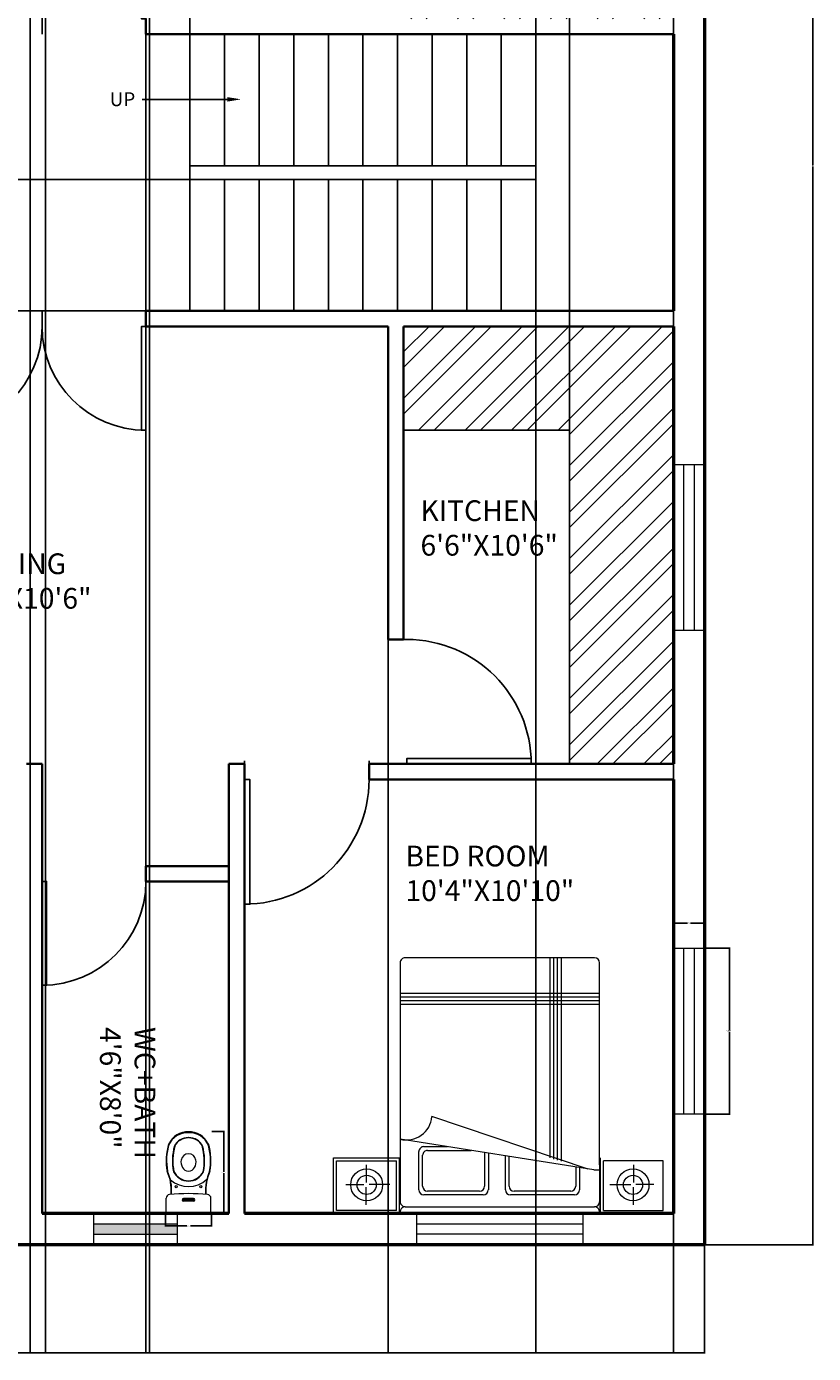
# Model space of a CAD drawing. Units: feet. Extents: x 2664 to 3060, y 1318 to 2005.
# Tile 2 of 5: x 2832 to 3060, y 1318 to 1702. Entities that reach past the tile are written whole.
import ezdxf
from ezdxf import colors
from ezdxf.entities.mleader import LeaderData, LeaderLine
from ezdxf.math import Vec2, Vec3

# ---------------------------------------------------------------- set-up
doc = ezdxf.new("R2010")
doc.units = ezdxf.units.FT
for name, color, linetype, lineweight in [('A-ANNO-DIMS', 2, 'Continuous', 18), ('A-ANNO-SYMB', 182, 'Continuous', 18), ('A-AREA-IDEN', 109, 'Continuous', 18), ('A-WALL-EXTR', 130, 'Continuous', 50), ('DOOR', 249, 'Continuous', 25), ('FURNITURE', 240, 'Continuous', 13), ('SANITARY', 50, 'Continuous', 13), ('STAIR', 182, 'Continuous', 25)]:
    doc.layers.add(name, color=color, linetype=linetype, lineweight=lineweight)
for name, color, linetype, lineweight, true_color in [('A-CASE', 41, 'Continuous', 25, 0xf5dd7a), ('A-CASE-PATT', 152, 'Continuous', 13, 0x2776bb), ('A-GLAZ', 222, 'Continuous', 18, 0xd4008b), ('A-VENT-PATT', 219, 'Continuous', 13, 0x642165), ('A-WALL-INTR', 41, 'Continuous', 35, 0xf5dd7a), ('VENT', 95, 'Continuous', 18, 0x46b72a)]:
    doc.layers.add(name, color=color, linetype=linetype, lineweight=lineweight, true_color=true_color)
doc.styles.get("Standard").update_dxf_attribs({"font": 'arial.ttf'})
doc.dimstyles.get("Standard").update_dxf_attribs({"dimtxt": 0.18, "dimasz": 0.18, "dimexe": 0.18, "dimexo": 0.0625, "dimgap": 0.09, "dimtad": 0, "dimtih": 1, "dimtoh": 1, "dimdec": 4, "dimzin": 0, "dimdsep": 46, "dimtxsty": 'Standard', "dimcen": 0.09, "dimadec": 0, "dimazin": 0, "dimtfac": 1, "dimtdec": 4, "dimtofl": 0, "dimtmove": 0, "dimatfit": 3, "dimfxl": 1, "dimtolj": 1, "dimtzin": 0, "dimarcsym": 0})

# ---------------------------------------------------------------- blocks, each defined once
blk = doc.blocks.new('*U4')
for p, q in [((0, 0), (0, 6)), ((40, 0), (40, 6))]:
    blk.add_line(p, q)
blk.add_lwpolyline([(0, 0), (0, -40), (1.75, -40), (1.75, 0)], close=True)
blk.add_arc((0, 0), 40, 270, 0)
blk = doc.blocks.new('*U3')
for p, q in [((0, 0), (0, -6)), ((-40, 0), (-40, -6))]:
    blk.add_line(p, q)
blk.add_lwpolyline([(0, 0), (0, 40), (-1.75, 40), (-1.75, 0)], close=True)
blk.add_arc((0, 0), 40, 90, 180)
blk = doc.blocks.new('*U7')
for p, q in [((0, 0), (0, 6)), ((40, 0), (40, 6))]:
    blk.add_line(p, q)
blk.add_lwpolyline([(0, 0), (0, -40), (1.75, -40), (1.75, 0)], close=True)
blk.add_arc((0, 0), 40, 270, 360)
blk = doc.blocks.new('*U2')
for p, q in [((0, 0), (0, -6)), ((40, 0), (40, -6))]:
    blk.add_line(p, q)
blk.add_lwpolyline([(0, 0), (0, 40), (1.75, 40), (1.75, 0)], close=True)
blk.add_arc((0, 0), 40, 0, 90)
blk = doc.blocks.new('*U6')
for p, q in [((0, 0), (0, 6)), ((40, 0), (40, 6))]:
    blk.add_line(p, q)
blk.add_lwpolyline([(0, 0), (0, -40), (1.75, -40), (1.75, 0)], close=True)
blk.add_arc((0, 0), 40, 270, 0)
blk = doc.blocks.new('BED-DOUBLE-WITH-NIGHTSTANDS')
for p, q in [((-29.54, 0), (-29.54, -16.21)), ((-30.37, -0.95), (-47.65, -0.95)), ((-47.65, -0.95), (-47.65, -15.35)), ((-39.11, -2.58), (-39.11, -7.74)), ((-30.37, -0.95), (-30.37, -15.35)), ((-29.47, -0.05), (-29.47, -16.25)), ((-29.26, -14.16), (-29.26, -3.5)), ((28.27, -0.11), (-29.17, -0.11)), ((26.92, -2.06), (-27.82, -2.06)), ((28.36, -72.65), (28.36, -3.5)), ((28.57, -0.05), (47.65, -0.05)), ((28.57, -0.05), (28.57, -16.25)), ((29.47, -0.95), (46.75, -0.95)), ((29.47, -0.95), (29.47, -15.35)), ((38.21, -2.58), (38.21, -7.74)), ((46.75, -0.95), (46.75, -15.35)), ((47.65, -0.05), (47.65, -16.25)), ((-23.45, -13.32), (-23.45, -6.94)), ((-22.01, -5.5), (-3.48, -5.5)), ((-20.93, -6.58), (-4.56, -6.58)), ((-2.04, -6.94), (-2.04, -16.8)), ((2.88, -17.58), (2.88, -6.94)), ((4.33, -5.5), (21.52, -5.5)), ((5.41, -6.58), (20.44, -6.58)), ((22.96, -6.94), (22.96, -18.02)), ((-44.95, -8.46), (-39.75, -8.46)), ((-39.11, -14.22), (-39.11, -9.06)), ((-32.27, -8.46), (-38.27, -8.46)), ((-22.37, -13.47), (-22.37, -8.02)), ((-3.12, -8.02), (-3.12, -16.63)), ((3.96, -17.76), (3.96, -8.02)), ((21.88, -8.02), (21.88, -16.94)), ((31.37, -8.46), (37.37, -8.46)), ((38.21, -14.22), (38.21, -9.06)), ((44.05, -8.46), (38.85, -8.46)), ((-27.62, -12.73), (-29.26, -12.73)), ((-29.26, -14.16), (-29.26, -72.65)), ((-27.62, -12.73), (28.36, -21.64)), ((-26, -12.96), (19.2, -28.15)), ((-18.14, -74.09), (-18.14, -15.24)), ((-47.65, -15.35), (-30.37, -15.35)), ((-17.06, -74.09), (-17.06, -15.55)), ((-15.97, -74.09), (-15.97, -15.86)), ((-14.89, -74.09), (-14.89, -16.18)), ((20.44, -18.38), (7.87, -18.38)), ((47.65, -16.25), (28.57, -16.25)), ((46.75, -15.35), (29.47, -15.35)), ((21.52, -19.46), (14.66, -19.46)), ((28.36, -60.64), (-29.26, -60.64)), ((28.36, -61.72), (-29.26, -61.72)), ((28.36, -62.8), (-29.26, -62.8)), ((28.36, -63.88), (-29.26, -63.88)), ((-27.82, -74.09), (26.92, -74.09))]:
    blk.add_line(p, q)
for centre, radius in [((-38.95, -8.4), 4.61), ((38.05, -8.4), 4.61), ((-38.95, -8.4), 2.77), ((38.05, -8.4), 2.77)]:
    blk.add_circle(centre, radius)
for centre, radius, start, end in [((-27.82, -0.62), 1.44, 159.2884, 270), ((-27.82, -3.5), 1.44, 90, 180), ((26.92, -0.62), 1.44, 270, 20.7116), ((26.92, -3.5), 1.44, 0, 90), ((-22.01, -6.94), 1.44, 90, 180), ((-20.93, -8.02), 1.44, 90, 180), ((-4.56, -8.02), 1.44, 0, 90), ((-3.48, -6.94), 1.44, 0, 90), ((4.33, -6.94), 1.44, 90, 180), ((5.41, -8.02), 1.44, 90, 180), ((20.44, -8.02), 1.44, 0, 90), ((21.52, -6.94), 1.44, 0, 90), ((20.44, -16.94), 1.44, 270, 0), ((21.52, -18.02), 1.44, 270, 0), ((26.5, -28.71), 7.32, 75.237, 175.5647), ((-27.82, -72.65), 1.44, 180, 270), ((26.92, -72.65), 1.44, 270, 0)]:
    blk.add_arc(centre, radius, start, end)
blk = doc.blocks.new('WC-FLOOR-MOUNT')
for p, q in [((-6.3, 0), (6.3, 0)), ((-6.48, -0.18), (-6.48, -4.43)), ((-1.44, -3.6), (1.44, -3.6)), ((-1.44, -3.71), (1.44, -3.71)), ((-1.44, -3.82), (-0.18, -3.82)), ((0.18, -3.82), (1.44, -3.82)), ((6.48, -0.18), (6.48, -4.43)), ((-1.44, -4.11), (-0.18, -4.11)), ((-1.44, -4.21), (1.44, -4.21)), ((-1.44, -4.32), (1.44, -4.32)), ((-0.07, -3.93), (-0.07, -4)), ((0.07, -3.93), (0.07, -4)), ((0.18, -4.11), (1.44, -4.11))]:
    blk.add_line(p, q)
for centre, radius in [((-3.57, -7.78), 0.318), ((-1.42, -3.96), 0.112), ((-1.42, -3.96), 0.0402), ((1.42, -3.96), 0.112), ((1.42, -3.96), 0.0402), ((3.57, -7.78), 0.318)]:
    blk.add_circle(centre, radius)
for centre, radius, start, end in [((-6.3, -0.18), 0.18, 90, 180), ((-1.44, -3.96), 0.36, 90, 180), ((-1.44, -3.96), 0.252, 90, 180), ((-1.44, -3.96), 0.144, 90, 270), ((-0.18, -3.93), 0.108, 0, 90), ((0.18, -3.93), 0.108, 90, 180), ((1.44, -3.96), 0.36, 0, 90), ((1.44, -3.96), 0.252, 0, 90), ((1.44, -3.96), 0.144, 270, 90), ((6.3, -0.18), 0.18, 0, 90), ((-5.4, -4.43), 1.08, 180, 264.6037), ((-17.58, -6.84), 12.59, 334.9634, 4.9109), ((-17.58, -6.84), 12.69, 334.9634, 4.9109), ((0, 52.77), 58.53, 264.6037, 275.3963), ((-1.44, -3.96), 0.36, 180, 270), ((-1.44, -3.96), 0.252, 180, 270), ((-0.18, -4), 0.108, 270, 0), ((0.18, -4), 0.108, 180, 270), ((1.44, -3.96), 0.36, 270, 0), ((1.44, -3.96), 0.252, 270, 0), ((17.58, -6.84), 12.69, 175.0891, 205.0366), ((17.58, -6.84), 12.59, 175.0891, 205.0366), ((5.4, -4.43), 1.08, 275.3963, 0), ((0.06, -15.51), 7.72, 48.0834, 133.5369), ((0, -14.17), 4.8, 25.6263, 154.3737), ((0, -14.17), 4.69, 25.6263, 154.3737), ((11.03, -15.28), 17.49, 169.7326, 196.2187), ((11.03, -15.28), 17.38, 169.7326, 196.2187), ((11.03, -15.28), 15.69, 168.2525, 195.7257), ((11.03, -15.28), 15.58, 168.2525, 196.2187), ((1.08, -14.97), 3.26, 149.7876, 189.0746), ((0, -14.17), 1.92, 25.6263, 154.3737), ((-1.08, -14.97), 3.26, 350.9254, 30.2124), ((-11.03, -15.28), 15.58, 344.3098, 11.7475), ((-11.03, -15.28), 15.69, 344.2743, 11.7475), ((-11.03, -15.28), 17.38, 343.7813, 10.2674), ((-11.03, -15.28), 17.49, 343.7813, 10.2674), ((0, -15.12), 2.16, 189.6495, 350.3505), ((-0.18, -17.24), 6.13, 204.3045, 271.6847), ((-0.18, -17.65), 6.02, 204.3045, 271.6847), ((-0.18, -17.65), 4.32, 205.8912, 271.6847), ((-0.18, -17.65), 4.22, 206.0212, 271.6847), ((0.18, -17.24), 6.13, 268.3153, 335.6955), ((0.18, -17.65), 6.02, 268.3153, 335.6955), ((0.18, -17.65), 4.32, 268.3153, 334.1088), ((0.18, -17.65), 4.22, 268.3153, 333.9788)]:
    blk.add_arc(centre, radius, start, end)
blk = doc.blocks.new('WINDOW-4FT')
for p, q in [((-24, 4.5), (24, 4.5)), ((-24, -4.5), (-24, 4.5)), ((24, 4.5), (24, -4.5)), ((-24, 1.5), (24, 1.5)), ((24, -1.5), (-24, -1.5)), ((24, -4.5), (-24, -4.5))]:
    blk.add_line(p, q)
blk = doc.blocks.new('*D18')
at = {"layer": 'A-ANNO-DIMS', "color": 0, "lineweight": -2, "transparency": 16777216}
for p, q in [((3028.34, 1435.35), (3035.66, 1435.35)), ((3035.48, 1435.17), (3035.48, 1411.53)), ((3035.48, 1387.53), (3035.48, 1411.16)), ((3028.34, 1387.35), (3035.66, 1387.35))]:
    blk.add_line(p, q, dxfattribs=at)
at = {"layer": 'A-ANNO-DIMS', "color": 0, "transparency": 16777216}
for points in [[(3035.45, 1435.17), (3035.51, 1435.17), (3035.48, 1435.35)], [(3035.45, 1387.53), (3035.51, 1387.53), (3035.48, 1387.35)]]:
    blk.add_solid(points, dxfattribs=at)
at = {"layer": 'Defpoints', "color": 0, "transparency": 16777216}
for p in [(3028.28, 1435.35), (3035.48, 1435.35), (3028.28, 1387.35)]:
    blk.add_point(p, dxfattribs=at)
at = {"layer": 'A-ANNO-DIMS', "color": 0, "transparency": 16777216, "insert": (3035.48, 1411.35), "char_height": 0.18, "attachment_point": 5}
blk.add_mtext('\\A1;WINDOW 48 TYP.', dxfattribs=at)
blk = doc.blocks.new('*D19')
at = {"layer": 'A-ANNO-DIMS', "color": 0, "lineweight": -2, "transparency": 16777216}
for p, q in [((3019.28, 1435.41), (3019.28, 1442.73)), ((3019.46, 1442.55), (3023.32, 1442.55)), ((3028.1, 1442.55), (3024.24, 1442.55)), ((3028.28, 1435.41), (3028.28, 1442.73))]:
    blk.add_line(p, q, dxfattribs=at)
at = {"layer": 'A-ANNO-DIMS', "color": 0, "transparency": 16777216}
for points in [[(3019.46, 1442.58), (3019.46, 1442.52), (3019.28, 1442.55)], [(3028.1, 1442.58), (3028.1, 1442.52), (3028.28, 1442.55)]]:
    blk.add_solid(points, dxfattribs=at)
at = {"layer": 'Defpoints', "color": 0, "transparency": 16777216}
for p in [(3019.28, 1442.55), (3019.28, 1435.35), (3028.28, 1435.35)]:
    blk.add_point(p, dxfattribs=at)
at = {"layer": 'A-ANNO-DIMS', "color": 0, "transparency": 16777216, "insert": (3023.78, 1442.55), "char_height": 0.18, "attachment_point": 5}
blk.add_mtext('\\A1;9 TYP.', dxfattribs=at)
blk = doc.blocks.new('*D30')
at = {"layer": 'A-ANNO-DIMS', "color": 0, "lineweight": -2, "transparency": 16777216}
for p, q in [((2885.83, 1382.31), (2889.51, 1382.31)), ((2889.33, 1382.13), (2889.33, 1370.62)), ((2889.33, 1358.75), (2889.33, 1370.25)), ((2885.83, 1358.57), (2889.51, 1358.57))]:
    blk.add_line(p, q, dxfattribs=at)
at = {"layer": 'A-ANNO-DIMS', "color": 0, "transparency": 16777216}
for points in [[(2889.3, 1382.13), (2889.36, 1382.13), (2889.33, 1382.31)], [(2889.3, 1358.75), (2889.36, 1358.75), (2889.33, 1358.57)]]:
    blk.add_solid(points, dxfattribs=at)
at = {"layer": 'Defpoints', "color": 0, "transparency": 16777216}
for p in [(2885.77, 1382.31), (2885.77, 1358.57), (2889.33, 1358.57)]:
    blk.add_point(p, dxfattribs=at)
at = {"layer": 'A-ANNO-DIMS', "color": 0, "transparency": 16777216, "insert": (2889.33, 1370.44), "char_height": 0.18, "attachment_point": 5}
blk.add_mtext('\\A1;WC 24 TYP.', dxfattribs=at)
blk = doc.blocks.new('*D31')
at = {"layer": 'A-ANNO-DIMS', "color": 0, "lineweight": -2, "transparency": 16777216}
for p, q in [((2872.44, 1358.51), (2872.44, 1354.83)), ((2885.77, 1358.51), (2885.77, 1354.83)), ((2872.62, 1355.01), (2878.59, 1355.01)), ((2885.59, 1355.01), (2879.63, 1355.01))]:
    blk.add_line(p, q, dxfattribs=at)
at = {"layer": 'A-ANNO-DIMS', "color": 0, "transparency": 16777216}
for points in [[(2872.62, 1355.04), (2872.62, 1354.98), (2872.44, 1355.01)], [(2885.59, 1355.04), (2885.59, 1354.98), (2885.77, 1355.01)]]:
    blk.add_solid(points, dxfattribs=at)
at = {"layer": 'Defpoints', "color": 0, "transparency": 16777216}
for p in [(2872.44, 1358.57), (2885.77, 1358.57), (2872.44, 1355.01)]:
    blk.add_point(p, dxfattribs=at)
at = {"layer": 'A-ANNO-DIMS', "color": 0, "transparency": 16777216, "insert": (2879.11, 1355.01), "char_height": 0.18, "attachment_point": 5}
blk.add_mtext('\\A1;13 TYP.', dxfattribs=at)
blk = doc.blocks.new('*D32')
at = {"layer": 'A-ANNO-DIMS', "color": 0, "lineweight": -2, "transparency": 16777216}
for p, q in [((2695.28, 1619.51), (2695.28, 1318.11)), ((3028.28, 1349.51), (3028.28, 1318.11)), ((2695.46, 1318.29), (2861.49, 1318.29)), ((3028.1, 1318.29), (2862.07, 1318.29))]:
    blk.add_line(p, q, dxfattribs=at)
at = {"layer": 'A-ANNO-DIMS', "color": 0, "transparency": 16777216}
for points in [[(2695.46, 1318.32), (2695.46, 1318.26), (2695.28, 1318.29)], [(3028.1, 1318.32), (3028.1, 1318.26), (3028.28, 1318.29)]]:
    blk.add_solid(points, dxfattribs=at)
at = {"layer": 'Defpoints', "color": 0, "transparency": 16777216}
for p in [(2695.28, 1619.57), (3028.28, 1349.57), (3028.28, 1318.29)]:
    blk.add_point(p, dxfattribs=at)
at = {"layer": 'A-ANNO-DIMS', "color": 0, "transparency": 16777216, "insert": (2861.78, 1318.29), "char_height": 0.18, "attachment_point": 5}
blk.add_mtext('\\A1;333', dxfattribs=at)
blk = doc.blocks.new('*D33')
at = {"layer": 'A-ANNO-DIMS', "color": 0, "lineweight": -2, "transparency": 16777216}
for p, q in [((3028.34, 1973.57), (3059.74, 1973.57)), ((3059.56, 1973.39), (3059.56, 1661.75)), ((3059.56, 1349.75), (3059.56, 1661.39)), ((3028.34, 1349.57), (3059.74, 1349.57))]:
    blk.add_line(p, q, dxfattribs=at)
at = {"layer": 'A-ANNO-DIMS', "color": 0, "transparency": 16777216}
for points in [[(3059.53, 1973.39), (3059.59, 1973.39), (3059.56, 1973.57)], [(3059.53, 1349.75), (3059.59, 1349.75), (3059.56, 1349.57)]]:
    blk.add_solid(points, dxfattribs=at)
at = {"layer": 'Defpoints', "color": 0, "transparency": 16777216}
for p in [(3028.28, 1973.57), (3059.56, 1973.57), (3028.28, 1349.57)]:
    blk.add_point(p, dxfattribs=at)
at = {"layer": 'A-ANNO-DIMS', "color": 0, "transparency": 16777216, "insert": (3059.56, 1661.57), "char_height": 0.18, "attachment_point": 5}
blk.add_mtext('\\A1;624', dxfattribs=at)
blk = doc.blocks.new('*D48')
at = {"layer": 'A-ANNO-DIMS', "color": 0, "lineweight": -2, "transparency": 16777216}
for p, q in [((2879.53, 1619.63), (2879.53, 2005.03)), ((2879.71, 2004.85), (2929.25, 2004.85)), ((2979.35, 2004.85), (2929.81, 2004.85)), ((2979.53, 1619.63), (2979.53, 2005.03))]:
    blk.add_line(p, q, dxfattribs=at)
at = {"layer": 'A-ANNO-DIMS', "color": 0, "transparency": 16777216}
for points in [[(2879.71, 2004.88), (2879.71, 2004.82), (2879.53, 2004.85)], [(2979.35, 2004.88), (2979.35, 2004.82), (2979.53, 2004.85)]]:
    blk.add_solid(points, dxfattribs=at)
at = {"layer": 'Defpoints', "color": 0, "transparency": 16777216}
for p in [(2979.53, 2004.85), (2879.53, 1619.57), (2979.53, 1619.57)]:
    blk.add_point(p, dxfattribs=at)
at = {"layer": 'A-ANNO-DIMS', "color": 0, "transparency": 16777216, "insert": (2929.53, 2004.85), "char_height": 0.18, "attachment_point": 5}
blk.add_mtext('\\A1;100', dxfattribs=at)
blk = doc.blocks.new('*D49')
at = {"layer": 'A-ANNO-DIMS', "color": 0, "lineweight": -2, "transparency": 16777216}
for p, q in [((2979.53, 1699.51), (2979.53, 1318.11)), ((3019.28, 1699.51), (3019.28, 1318.11)), ((2979.71, 1318.29), (2999.01, 1318.29)), ((3019.1, 1318.29), (2999.8, 1318.29))]:
    blk.add_line(p, q, dxfattribs=at)
at = {"layer": 'A-ANNO-DIMS', "color": 0, "transparency": 16777216}
for points in [[(2979.71, 1318.32), (2979.71, 1318.26), (2979.53, 1318.29)], [(3019.1, 1318.32), (3019.1, 1318.26), (3019.28, 1318.29)]]:
    blk.add_solid(points, dxfattribs=at)
at = {"layer": 'Defpoints', "color": 0, "transparency": 16777216}
for p in [(2979.53, 1699.57), (3019.28, 1699.57), (3019.28, 1318.29)]:
    blk.add_point(p, dxfattribs=at)
at = {"layer": 'A-ANNO-DIMS', "color": 0, "transparency": 16777216, "insert": (2999.41, 1318.29), "char_height": 0.18, "attachment_point": 5}
blk.add_mtext('\\A1;39.75', dxfattribs=at)
blk = doc.blocks.new('*D50')
at = {"layer": 'A-ANNO-DIMS', "color": 0, "lineweight": -2, "transparency": 16777216}
for p, q in [((2879.47, 1657.57), (2663.82, 1657.57)), ((2664, 1657.39), (2664, 1638.75)), ((2664, 1619.75), (2664, 1638.39)), ((2879.47, 1619.57), (2663.82, 1619.57))]:
    blk.add_line(p, q, dxfattribs=at)
at = {"layer": 'A-ANNO-DIMS', "color": 0, "transparency": 16777216}
for points in [[(2663.97, 1657.39), (2664.03, 1657.39), (2664, 1657.57)], [(2663.97, 1619.75), (2664.03, 1619.75), (2664, 1619.57)]]:
    blk.add_solid(points, dxfattribs=at)
at = {"layer": 'Defpoints', "color": 0, "transparency": 16777216}
for p in [(2664, 1657.57), (2879.53, 1657.57), (2879.53, 1619.57)]:
    blk.add_point(p, dxfattribs=at)
at = {"layer": 'A-ANNO-DIMS', "color": 0, "transparency": 16777216, "insert": (2664, 1638.57), "char_height": 0.18, "attachment_point": 5}
blk.add_mtext('\\A1;38', dxfattribs=at)
blk = doc.blocks.new('*D51')
at = {"layer": 'A-ANNO-DIMS', "color": 0, "lineweight": -2, "transparency": 16777216}
for p, q in [((2806.78, 1699.51), (2806.78, 1318.11)), ((2866.78, 1699.51), (2866.78, 1318.11)), ((2806.96, 1318.29), (2836.56, 1318.29)), ((2866.6, 1318.29), (2837, 1318.29))]:
    blk.add_line(p, q, dxfattribs=at)
at = {"layer": 'A-ANNO-DIMS', "color": 0, "transparency": 16777216}
for points in [[(2806.96, 1318.32), (2806.96, 1318.26), (2806.78, 1318.29)], [(2866.6, 1318.32), (2866.6, 1318.26), (2866.78, 1318.29)]]:
    blk.add_solid(points, dxfattribs=at)
at = {"layer": 'Defpoints', "color": 0, "transparency": 16777216}
for p in [(2806.78, 1699.57), (2866.78, 1699.57), (2866.78, 1318.29)]:
    blk.add_point(p, dxfattribs=at)
at = {"layer": 'A-ANNO-DIMS', "color": 0, "transparency": 16777216, "insert": (2836.78, 1318.29), "char_height": 0.18, "attachment_point": 5}
blk.add_mtext('\\A1;60', dxfattribs=at)
blk = doc.blocks.new('*D52')
at = {"layer": 'A-ANNO-DIMS', "color": 0, "lineweight": -2, "transparency": 16777216}
for p, q in [((2866.78, 1615.01), (2866.78, 1318.11)), ((2936.78, 1615.01), (2936.78, 1318.11)), ((2866.96, 1318.29), (2901.56, 1318.29)), ((2936.6, 1318.29), (2902, 1318.29))]:
    blk.add_line(p, q, dxfattribs=at)
at = {"layer": 'A-ANNO-DIMS', "color": 0, "transparency": 16777216}
for points in [[(2866.96, 1318.32), (2866.96, 1318.26), (2866.78, 1318.29)], [(2936.6, 1318.32), (2936.6, 1318.26), (2936.78, 1318.29)]]:
    blk.add_solid(points, dxfattribs=at)
at = {"layer": 'Defpoints', "color": 0, "transparency": 16777216}
for p in [(2866.78, 1615.07), (2936.78, 1615.07), (2936.78, 1318.29)]:
    blk.add_point(p, dxfattribs=at)
at = {"layer": 'A-ANNO-DIMS', "color": 0, "transparency": 16777216, "insert": (2901.78, 1318.29), "char_height": 0.18, "attachment_point": 5}
blk.add_mtext('\\A1;70', dxfattribs=at)
blk = doc.blocks.new('*D53')
at = {"layer": 'A-ANNO-DIMS', "color": 0, "lineweight": -2, "transparency": 16777216}
for p, q in [((2797.28, 1830.01), (2797.28, 1318.11)), ((2833.28, 1830.01), (2833.28, 1318.11)), ((2797.46, 1318.29), (2815.06, 1318.29)), ((2833.1, 1318.29), (2815.5, 1318.29))]:
    blk.add_line(p, q, dxfattribs=at)
at = {"layer": 'A-ANNO-DIMS', "color": 0, "transparency": 16777216}
for points in [[(2797.46, 1318.32), (2797.46, 1318.26), (2797.28, 1318.29)], [(2833.1, 1318.32), (2833.1, 1318.26), (2833.28, 1318.29)]]:
    blk.add_solid(points, dxfattribs=at)
at = {"layer": 'Defpoints', "color": 0, "transparency": 16777216}
for p in [(2797.28, 1830.07), (2833.28, 1830.07), (2833.28, 1318.29)]:
    blk.add_point(p, dxfattribs=at)
at = {"layer": 'A-ANNO-DIMS', "color": 0, "transparency": 16777216, "insert": (2815.28, 1318.29), "char_height": 0.18, "attachment_point": 5}
blk.add_mtext('\\A1;36', dxfattribs=at)
blk = doc.blocks.new('*D54')
at = {"layer": 'A-ANNO-DIMS', "color": 0, "lineweight": -2, "transparency": 16777216}
for p, q in [((2837.78, 1868.51), (2837.78, 1318.11)), ((2867.78, 1868.51), (2867.78, 1318.11)), ((2837.96, 1318.29), (2852.56, 1318.29)), ((2867.6, 1318.29), (2853, 1318.29))]:
    blk.add_line(p, q, dxfattribs=at)
at = {"layer": 'A-ANNO-DIMS', "color": 0, "transparency": 16777216}
for points in [[(2837.96, 1318.32), (2837.96, 1318.26), (2837.78, 1318.29)], [(2867.6, 1318.32), (2867.6, 1318.26), (2867.78, 1318.29)]]:
    blk.add_solid(points, dxfattribs=at)
at = {"layer": 'Defpoints', "color": 0, "transparency": 16777216}
for p in [(2837.78, 1868.57), (2867.78, 1868.57), (2867.78, 1318.29)]:
    blk.add_point(p, dxfattribs=at)
at = {"layer": 'A-ANNO-DIMS', "color": 0, "transparency": 16777216, "insert": (2852.78, 1318.29), "char_height": 0.18, "attachment_point": 5}
blk.add_mtext('\\A1;30', dxfattribs=at)
blk = doc.blocks.new('*D55')
at = {"layer": 'A-ANNO-DIMS', "color": 0, "lineweight": -2, "transparency": 16777216}
for p, q in [((2833.28, 1830.01), (2833.28, 1318.11)), ((2837.78, 1830.01), (2837.78, 1318.11)), ((2833.46, 1318.29), (2835.27, 1318.29)), ((2837.6, 1318.29), (2835.79, 1318.29))]:
    blk.add_line(p, q, dxfattribs=at)
at = {"layer": 'A-ANNO-DIMS', "color": 0, "transparency": 16777216}
for points in [[(2833.46, 1318.32), (2833.46, 1318.26), (2833.28, 1318.29)], [(2837.6, 1318.32), (2837.6, 1318.26), (2837.78, 1318.29)]]:
    blk.add_solid(points, dxfattribs=at)
at = {"layer": 'Defpoints', "color": 0, "transparency": 16777216}
for p in [(2833.28, 1830.07), (2837.78, 1830.07), (2837.78, 1318.29)]:
    blk.add_point(p, dxfattribs=at)
at = {"layer": 'A-ANNO-DIMS', "color": 0, "transparency": 16777216, "insert": (2835.53, 1318.29), "char_height": 0.18, "attachment_point": 5}
blk.add_mtext('\\A1;4.5', dxfattribs=at)
blk = doc.blocks.new('*D58')
at = {"layer": 'A-ANNO-DIMS', "color": 0, "lineweight": -2, "transparency": 16777216}
for p, q in [((2989.28, 1488.63), (2989.28, 2005.03)), ((2989.46, 2004.85), (3004.06, 2004.85)), ((3019.1, 2004.85), (3004.5, 2004.85)), ((3019.28, 1488.63), (3019.28, 2005.03))]:
    blk.add_line(p, q, dxfattribs=at)
at = {"layer": 'A-ANNO-DIMS', "color": 0, "transparency": 16777216}
for points in [[(2989.46, 2004.88), (2989.46, 2004.82), (2989.28, 2004.85)], [(3019.1, 2004.88), (3019.1, 2004.82), (3019.28, 2004.85)]]:
    blk.add_solid(points, dxfattribs=at)
at = {"layer": 'Defpoints', "color": 0, "transparency": 16777216}
for p in [(3019.28, 2004.85), (2989.28, 1488.57), (3019.28, 1488.57)]:
    blk.add_point(p, dxfattribs=at)
at = {"layer": 'A-ANNO-DIMS', "color": 0, "transparency": 16777216, "insert": (3004.28, 2004.85), "char_height": 0.18, "attachment_point": 5}
blk.add_mtext('\\A1;30', dxfattribs=at)

msp = doc.modelspace()

# ---------------------------------------------------------------- hatches: boundary and pattern name
at = {"layer": 'A-CASE-PATT'}
h = msp.add_hatch(dxfattribs=at)
h.set_pattern_fill('ANSI32', color=256)
h.paths.add_polyline_path([(3019.28, 1615.071), (2941.28, 1615.071), (2941.28, 1585.071), (2989.28, 1585.071), (2989.28, 1488.571), (3019.28, 1488.571)])
h.paths.add_polyline_path([(3019.28, 1830.071), (2995.28, 1830.071), (2995.28, 1734.071), (2941.28, 1734.071), (2941.28, 1704.071), (3019.28, 1704.071)])
at = {"layer": 'A-VENT-PATT'}
h = msp.add_hatch(color=256, dxfattribs=at)
h.dxf.hatch_style = 1
h.paths.add_polyline_path([(2875.78, 1352.571), (2875.78, 1355.571), (2851.78, 1355.571), (2851.78, 1352.571)])

# ---------------------------------------------------------------- linework, layer by layer
at = {"layer": 'A-CASE'}
for p, q in [((2941.28, 1585.071), (2989.28, 1585.071)), ((2989.28, 1585.071), (2989.28, 1488.571))]:
    msp.add_line(p, q, dxfattribs=at)
at = {"layer": 'A-WALL-EXTR'}
for p, q in [((3028.28, 1973.571), (3028.28, 1349.571)), ((3019.28, 1699.571), (3019.28, 1619.571)), ((3019.28, 1615.071), (3019.28, 1488.571)), ((3019.28, 1484.071), (3019.28, 1358.571)), ((2890.78, 1358.571), (2836.78, 1358.571)), ((3019.28, 1358.571), (2895.28, 1358.571)), ((3028.28, 1349.571), (2704.28, 1349.571))]:
    msp.add_line(p, q, dxfattribs=at)
at = {"layer": 'A-WALL-INTR'}
for p, q in [((2866.78, 1699.571), (2866.78, 1704.071)), ((3019.28, 1699.571), (2866.78, 1699.571)), ((2866.78, 1615.071), (2866.78, 1619.571)), ((2866.78, 1619.571), (3019.28, 1619.571)), ((2866.78, 1615.071), (2936.78, 1615.071)), ((2936.78, 1615.071), (2936.78, 1524.571)), ((2941.28, 1615.071), (2941.28, 1524.571)), ((2941.28, 1615.071), (3019.28, 1615.071)), ((2936.78, 1524.571), (2941.28, 1524.571)), ((2836.78, 1488.571), (2832.28, 1488.571)), ((2836.78, 1488.571), (2836.78, 1358.571)), ((2890.78, 1488.571), (2890.78, 1358.571)), ((2895.28, 1488.571), (2890.78, 1488.571)), ((2895.28, 1488.571), (2895.28, 1358.571)), ((2936.78, 1488.571), (2931.28, 1488.571)), ((2931.28, 1488.571), (2931.28, 1484.071)), ((2936.78, 1488.571), (2941.28, 1488.571)), ((3019.28, 1488.571), (2941.28, 1488.571)), ((3019.28, 1484.071), (2931.28, 1484.071)), ((2890.78, 1459.071), (2866.78, 1459.071)), ((2866.78, 1459.071), (2866.78, 1454.571)), ((2890.78, 1454.571), (2866.78, 1454.571))]:
    msp.add_line(p, q, dxfattribs=at)
at = {"layer": 'STAIR'}
for p, q in [((2879.53, 1699.571), (2879.53, 1619.571)), ((2889.53, 1699.571), (2889.53, 1661.571)), ((2899.53, 1699.571), (2899.53, 1661.571)), ((2909.53, 1699.571), (2909.53, 1661.571)), ((2919.53, 1699.571), (2919.53, 1661.571)), ((2929.53, 1699.571), (2929.53, 1661.571)), ((2939.53, 1699.571), (2939.53, 1661.571)), ((2949.53, 1699.571), (2949.53, 1661.571)), ((2959.53, 1699.571), (2959.53, 1661.571)), ((2969.53, 1699.571), (2969.53, 1661.571)), ((2979.53, 1699.571), (2979.53, 1619.571)), ((2979.53, 1661.571), (2879.53, 1661.571)), ((2979.53, 1657.571), (2879.53, 1657.571)), ((2889.53, 1657.571), (2889.53, 1619.571)), ((2899.53, 1657.571), (2899.53, 1619.571)), ((2909.53, 1657.571), (2909.53, 1619.571)), ((2919.53, 1657.571), (2919.53, 1619.571)), ((2929.53, 1657.571), (2929.53, 1619.571)), ((2939.53, 1657.571), (2939.53, 1619.571)), ((2949.53, 1657.571), (2949.53, 1619.571)), ((2959.53, 1657.571), (2959.53, 1619.571)), ((2969.53, 1657.571), (2969.53, 1619.571)), ((2866.78, 1619.571), (2936.78, 1619.571))]:
    msp.add_line(p, q, dxfattribs=at)
at = {"layer": 'VENT'}
for p, q in [((2851.78, 1358.571), (2875.78, 1358.571)), ((2851.78, 1349.571), (2851.78, 1358.571)), ((2875.78, 1358.571), (2875.78, 1349.571)), ((2851.78, 1355.571), (2875.78, 1355.571)), ((2851.78, 1352.571), (2875.78, 1352.571)), ((2875.78, 1349.571), (2851.78, 1349.571))]:
    msp.add_line(p, q, dxfattribs=at)

# ---------------------------------------------------------------- block references
at = {"layer": 'A-GLAZ'}
for p, rotation in [((3023.78, 1551.15), 89.99999999999864), ((3023.78, 1411.348), 89.99999999999864), ((2969.111, 1354.071), 180)]:
    msp.add_blockref('WINDOW-4FT', p, dxfattribs=dict(at, rotation=rotation))
at = {"layer": 'DOOR'}
for name, p, xscale, yscale, zscale in [('*U2', (2806.78, 1704.071), 0.7500000000000038, 0.7500000000000038, 0.7500000000000038), ('*U2', (2866.78, 1704.071), -0.7500000000000038, 0.7500000000000038, 0.7500000000000038), ('*U6', (2806.78, 1615.071), 0.7500000000000038, 0.7500000000000038, 0.7500000000000038), ('*U6', (2866.78, 1615.071), -0.7500000000000038, 0.7500000000000038, 0.7500000000000038), ('*U4', (2895.28, 1484.044), 0.899999999999959, 0.899999999999959, 0.899999999999959), ('*U7', (2836.78, 1454.601), 0.7500000000000038, 0.7500000000000038, 0.7500000000000038)]:
    msp.add_blockref(name, p, dxfattribs=dict(at, xscale=xscale, yscale=yscale, zscale=zscale))
at = {"layer": 'DOOR', "xscale": 0.899999999999959, "yscale": 0.899999999999959, "zscale": 0.899999999999959, "rotation": 270}
msp.add_blockref('*U3', (2942.18, 1488.571), dxfattribs=at)
at = {"layer": 'FURNITURE', "rotation": 180}
msp.add_blockref('BED-DOUBLE-WITH-NIGHTSTANDS', (2968.661, 1358.464), dxfattribs=at)
at = {"layer": 'SANITARY', "rotation": 180}
msp.add_blockref('WC-FLOOR-MOUNT', (2879.106, 1358.571), dxfattribs=at)

# ---------------------------------------------------------------- texts
at = {"layer": 'A-AREA-IDEN', "char_height": 6, "attachment_point": 1}
for s, width, insert in [('KITCHEN\\P6\'6"X10\'6"', 22.955, (2946.163, 1564.821)), ('DRAWING \\P18\'8"X10\'6"', 22.955, (2806.796, 1549.47)), ('BED ROOM \\P10\'4"X10\'10"', 44.83878, (2941.807, 1464.949))]:
    msp.add_mtext_dynamic_manual_height_columns(s, width=width, gutter_width=12.5, heights=[0], dxfattribs=dict(at, insert=insert))
at = {"layer": 'A-AREA-IDEN', "insert": (2869.507, 1412.521), "char_height": 6, "attachment_point": 1, "rotation": 270}
msp.add_mtext_dynamic_manual_height_columns('WC+BATH\\P4\'6"X8\'0"', width=40.41148, gutter_width=12.5, heights=[0], dxfattribs=at)

# ---------------------------------------------------------------- dimensions: what is measured, and where the dimension line sits
at = {"layer": 'A-ANNO-DIMS'}
for base, p1, p2, override, picture, middle in [((2979.53, 2004.851), (2879.53, 1619.571), (2979.53, 1619.571), {"dimdec": 0, "dimlfac": 1, "dimrnd": 0, "dimzin": 0, "dimdsep": 46, "dimlunit": 2}, '*D48', (2929.53, 2004.851)), ((3019.28, 2004.851), (2989.28, 1488.571), (3019.28, 1488.571), {"dimdec": 0, "dimlfac": 1, "dimrnd": 0, "dimzin": 0, "dimdsep": 46, "dimlunit": 2}, '*D58', (3004.28, 2004.851)), ((2867.78, 1318.291), (2837.78, 1868.571), (2867.78, 1868.571), {"dimdec": 0, "dimlfac": 1, "dimrnd": 0, "dimzin": 0, "dimdsep": 46, "dimlunit": 2}, '*D54', (2852.78, 1318.291)), ((2833.28, 1318.291), (2797.28, 1830.071), (2833.28, 1830.071), {"dimdec": 0, "dimlfac": 1, "dimrnd": 0, "dimzin": 0, "dimdsep": 46, "dimlunit": 2}, '*D53', (2815.28, 1318.291)), ((2837.78, 1318.291), (2833.28, 1830.071), (2837.78, 1830.071), {"dimdec": 1, "dimlfac": 1, "dimrnd": 0, "dimzin": 0, "dimdsep": 46, "dimlunit": 2}, '*D55', (2835.53, 1318.291)), ((2866.78, 1318.291), (2806.78, 1699.571), (2866.78, 1699.571), {"dimdec": 0, "dimlfac": 1, "dimrnd": 0, "dimzin": 0, "dimdsep": 46, "dimlunit": 2}, '*D51', (2836.78, 1318.291)), ((3019.28, 1318.291), (2979.53, 1699.571), (3019.28, 1699.571), {"dimdec": 2, "dimlfac": 1, "dimrnd": 0, "dimzin": 0, "dimdsep": 46, "dimlunit": 2}, '*D49', (2999.405, 1318.291)), ((3028.28, 1318.291), (2695.28, 1619.571), (3028.28, 1349.571), {"dimdec": 0, "dimlfac": 1, "dimrnd": 0, "dimzin": 0, "dimdsep": 46, "dimlunit": 2}, '*D32', (2861.78, 1318.291)), ((2936.78, 1318.291), (2866.78, 1615.071), (2936.78, 1615.071), {"dimdec": 0, "dimlfac": 1, "dimrnd": 0, "dimzin": 0, "dimdsep": 46, "dimlunit": 2}, '*D52', (2901.78, 1318.291))]:
    dim = msp.add_linear_dim(base=base, p1=p1, p2=p2, dimstyle='Standard', override=override, dxfattribs=at)
    dim.commit()
    dim.dimension.update_dxf_attribs({"geometry": picture, "text_midpoint": middle})
for base, p1, p2, picture, middle in [((3059.56, 1973.571), (3028.28, 1349.571), (3028.28, 1973.571), '*D33', (3059.56, 1661.571)), ((2664, 1657.571), (2879.53, 1619.571), (2879.53, 1657.571), '*D50', (2664, 1638.571))]:
    dim = msp.add_linear_dim(base=base, p1=p1, p2=p2, angle=90, dimstyle='Standard', override={"dimdec": 0, "dimlfac": 1, "dimrnd": 0, "dimzin": 0, "dimdsep": 46, "dimlunit": 2}, dxfattribs=at)
    dim.commit()
    dim.dimension.update_dxf_attribs({"geometry": picture, "text_midpoint": middle})
for base, p1, p2, angle, text, picture, middle in [((3019.28, 1442.548), (3028.28, 1435.348), (3019.28, 1435.348), 180, '<> TYP.', '*D19', (3023.78, 1442.548)), ((3035.48, 1435.348), (3028.28, 1387.348), (3028.28, 1435.348), 90, 'WINDOW <> TYP.', '*D18', (3035.48, 1411.348)), ((2889.327, 1358.571), (2885.767, 1382.305), (2885.767, 1358.571), 270, 'WC <> TYP.', '*D30', (2889.327, 1370.438)), ((2872.444, 1355.01), (2885.767, 1358.571), (2872.444, 1358.571), 180, '<> TYP.', '*D31', (2879.106, 1355.01))]:
    dim = msp.add_linear_dim(base=base, p1=p1, p2=p2, angle=angle, text=text, dimstyle='Standard', override={"dimdec": 0, "dimlfac": 1, "dimrnd": 0, "dimzin": 0, "dimdsep": 46, "dimlunit": 2}, dxfattribs=at)
    dim.commit()
    dim.dimension.update_dxf_attribs({"geometry": picture, "text_midpoint": middle})

# ---------------------------------------------------------------- leaders
at = {"layer": 'A-ANNO-SYMB'}
ml = msp.add_multileader_mtext('Standard', dxfattribs=at)
ml.set_content('UP', color=256)
ml.set_leader_properties()
ml.build(insert=Vec2(0, 0))
ctx = ml.context
ctx.base_point, ctx.plane_origin = Vec3(2854.626, 1680.767), Vec3(2894.282, 1680.767)
ctx.text_align_type = 2
notes = []
notes.append((ctx, [(0, (1, 1, 0), (2873.707, 1680.767), (-1, 0), 8, [(0, [(2894.282, 1680.767)], 0, [])])]))
ctx.mtext.insert, ctx.mtext.alignment, ctx.mtext.flow_direction = Vec3(2863.707, 1682.801), 3, 5
for ctx, leaders in notes:
    for number, flags, end, landing, length, lines in leaders:
        leader = LeaderData()
        leader.index, (leader.has_last_leader_line, leader.has_dogleg_vector, leader.attachment_direction) = number, flags
        leader.last_leader_point, leader.dogleg_vector, leader.dogleg_length = Vec3(end), Vec3(landing), length
        for number, points, colour, breaks in lines:
            line = LeaderLine()
            line.index, line.vertices, line.color, line.breaks = number, Vec3.list(points), colors.encode_raw_color(colour), breaks
            leader.lines.append(line)
        ctx.leaders.append(leader)

doc.saveas('drawing.dxf')
